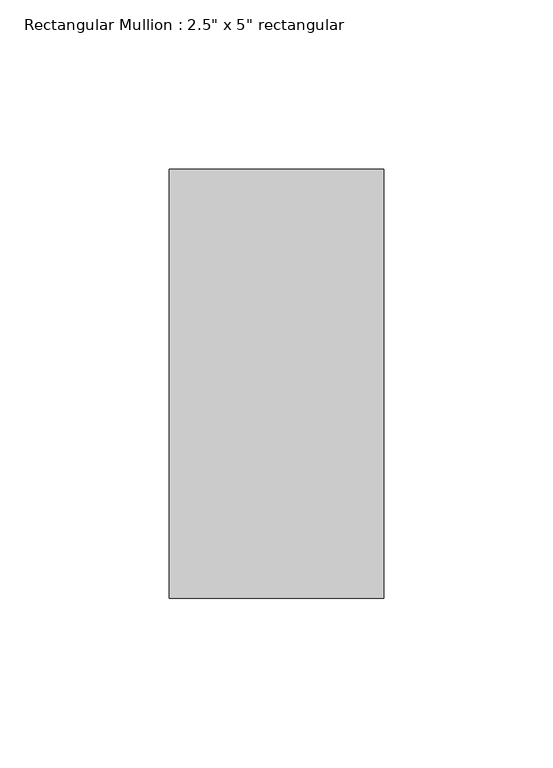
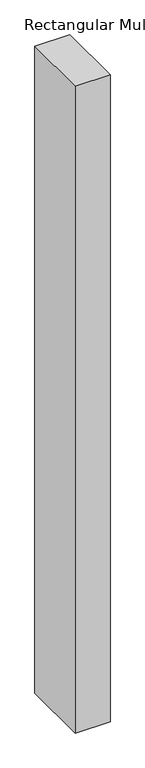
"""IFC4 building model written with IfcOpenShell, lengths in millimetres: member geometry."""

from ifc_helpers import new_model, si_unit, frame, origin, place, context, project, spatial, polyline, outline, extrude, source, transform, mapped, element, save


def member_a1da5be3(model_context):
    return source(origin(), model_context, "Body", "SweptSolid", [
        extrude(outline(polyline([(31.75, 63.5), (31.75, -63.5), (-31.75, -63.5), (-31.75, 63.5), (31.75, 63.5)])), frame((0.0, 0.0, -1244.6), z_axis=(0.0, 0.0, 1.0), x_axis=(1.0, 0.0, 0.0)), (0.0, 0.0, 1.0), 1244.6),
    ])


if __name__ == "__main__":
    model = new_model("IFC4")
    model_context = context("Model", 3, world=origin())
    ifc_project = project(units=[si_unit("LENGTHUNIT", "METRE", prefix="MILLI")], contexts=[model_context])
    site = spatial("IfcSite", under=ifc_project)
    building = spatial("IfcBuilding", under=site)
    placement = place(None, origin())
    member_shape = member_a1da5be3(model_context)
    element("IfcMember", 1, ObjectType="Rectangular Mullion : 2.5\" x 5\" rectangular", at=placement, inside=building, context=model_context, shape_type="MappedRepresentation", body=[
        mapped(member_shape, transform((0.0, 0.0, 0.0), x_axis=(1.0, 0.0, 0.0), y_axis=(0.0, 1.0, 0.0), z_axis=(0.0, 0.0, 1.0))),
    ])
    save(model, "model.ifc")

# Revit data of these elements
# Type "Rectangular Mullion : 2.5\" x 5\" rectangular"
#   built-in parameter 1007304 = 0.416667 (stored number, unit not read)
#   built-in parameter 1007301 = 0.104167 (stored number, unit not read)
#   built-in parameter 1007300 = 0.104167 (stored number, unit not read)
# Element 1 (IfcMember, "Rectangular Mullion : 2.5\" x 5\" rectangular")
#   Materials on its faces: "Aluminum"
# Materials
#   "Aluminum": class "Metal", colour RGB 247 247 247, transparency 0, Description = "Aluminum 6061", Cost = 0
